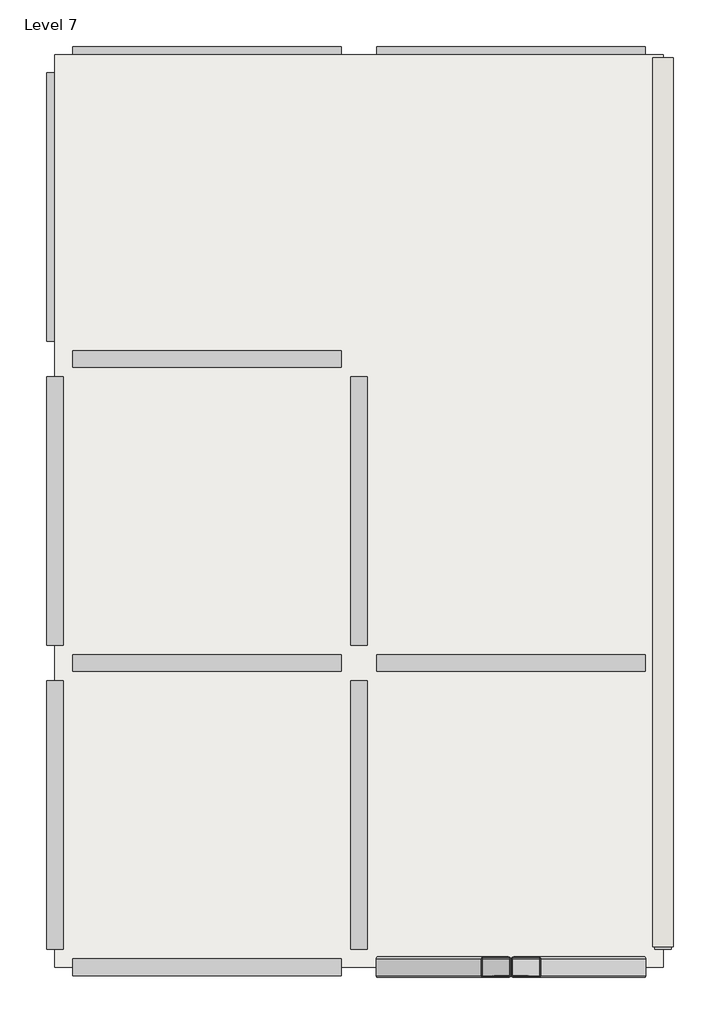
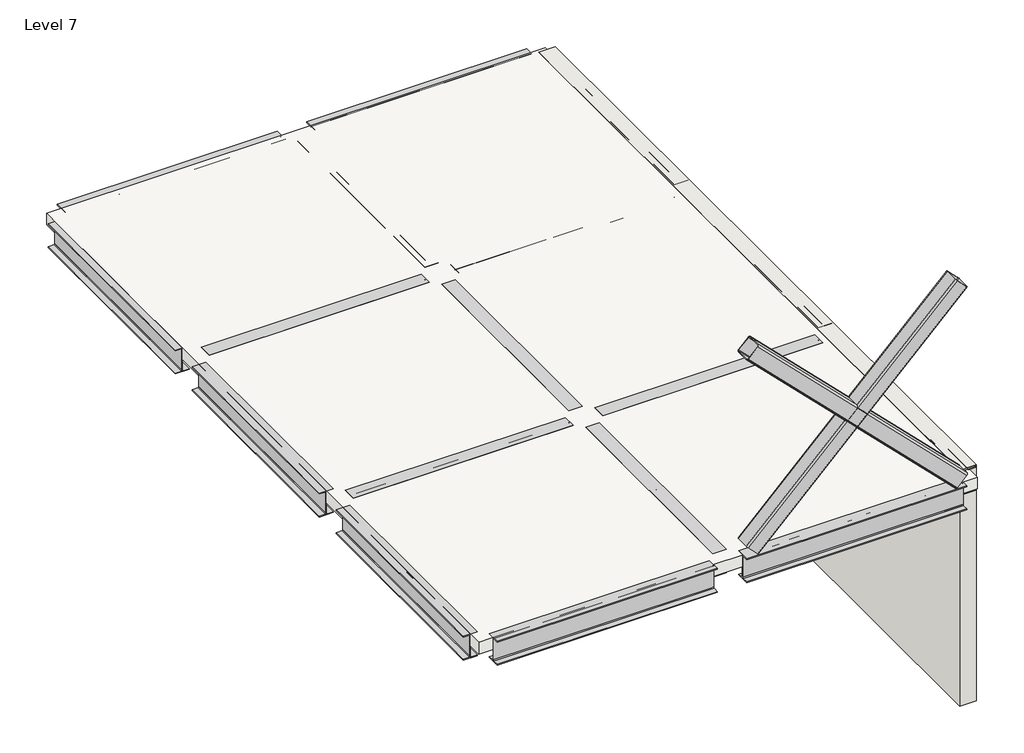
# One storey: 17 beams, 2 members, 1 slab, 1 wall.
"""IFC4 building model written with IfcOpenShell, lengths in millimetres."""

from ifc_helpers import new_model, si_unit, frame, origin, place, context, project, spatial, polyline, outline, extrude, transform, mapped, element, save
from components import ub_universal_beams_ub305x165x40_60ab2ee1, m_hss_square_hss203_2x203_2x9_5_07d005dd

model = new_model("IFC4")

# Units and contexts
model_context = context("Model", 3, world=origin())
ifc_project = project(units=[si_unit("LENGTHUNIT", "METRE", prefix="MILLI")], contexts=[model_context])

# Site, building, storey
site = spatial("IfcSite", under=ifc_project)
building = spatial("IfcBuilding", under=site)
storey = spatial("IfcBuildingStorey", under=building, Name="Level 7", Elevation=18000.0)

# Beams
placement = place(None, origin())
ub_universal_beams_ub305x165x40_shape = ub_universal_beams_ub305x165x40_60ab2ee1(model_context)
element("IfcBeam", 1, ObjectType="UB-Universal Beams : UB305x165x40", at=placement, inside=storey, context=model_context, shape_type="MappedRepresentation", body=[
    mapped(ub_universal_beams_ub305x165x40_shape, transform((18435.1404262, -6314.7314166, 17848.3), x_axis=(-1.0, 0.0, 0.0), y_axis=(0.0, -1.0, 0.0), z_axis=(0.0, 0.0, 1.0))),
])
element("IfcBeam", 2, ObjectType="UB-Universal Beams : UB305x165x40", at=placement, inside=storey, context=model_context, shape_type="MappedRepresentation", body=[
    mapped(ub_universal_beams_ub305x165x40_shape, transform((15435.1404262, -6314.7314166, 17848.3), x_axis=(-1.0, 0.0, 0.0), y_axis=(0.0, -1.0, 0.0), z_axis=(0.0, 0.0, 1.0))),
])
element("IfcBeam", 3, ObjectType="UB-Universal Beams : UB305x165x40", at=placement, inside=storey, context=model_context, shape_type="MappedRepresentation", body=[
    mapped(ub_universal_beams_ub305x165x40_shape, transform((13935.1404262, -4814.7314166, 17848.3), x_axis=(0.0, 1.0, 0.0), y_axis=(-1.0, 0.0, 0.0), z_axis=(0.0, 0.0, 1.0))),
])
element("IfcBeam", 4, ObjectType="UB-Universal Beams : UB305x165x40", at=placement, inside=storey, context=model_context, shape_type="MappedRepresentation", body=[
    mapped(ub_universal_beams_ub305x165x40_shape, transform((13935.1404262, -1814.7314166, 17848.3), x_axis=(0.0, 1.0, 0.0), y_axis=(-1.0, 0.0, 0.0), z_axis=(0.0, 0.0, 1.0))),
])
element("IfcBeam", 5, ObjectType="UB-Universal Beams : UB305x165x40", at=placement, inside=storey, context=model_context, shape_type="MappedRepresentation", body=[
    mapped(ub_universal_beams_ub305x165x40_shape, transform((13935.1404262, 1185.2685834, 17848.3), x_axis=(0.0, 1.0, 0.0), y_axis=(-1.0, 0.0, 0.0), z_axis=(0.0, 0.0, 1.0))),
])
element("IfcBeam", 6, ObjectType="UB-Universal Beams : UB305x165x40", at=placement, inside=storey, context=model_context, shape_type="MappedRepresentation", body=[
    mapped(ub_universal_beams_ub305x165x40_shape, transform((18435.1404262, -3314.7314166, 17848.3), x_axis=(-1.0, 0.0, 0.0), y_axis=(0.0, -1.0, 0.0), z_axis=(0.0, 0.0, 1.0))),
])
element("IfcBeam", 7, ObjectType="UB-Universal Beams : UB305x165x40", at=placement, inside=storey, context=model_context, shape_type="MappedRepresentation", body=[
    mapped(ub_universal_beams_ub305x165x40_shape, transform((15435.1404262, -3314.7314166, 17848.3), x_axis=(-1.0, 0.0, 0.0), y_axis=(0.0, -1.0, 0.0), z_axis=(0.0, 0.0, 1.0))),
])
element("IfcBeam", 8, ObjectType="UB-Universal Beams : UB305x165x40", at=placement, inside=storey, context=model_context, shape_type="MappedRepresentation", body=[
    mapped(ub_universal_beams_ub305x165x40_shape, transform((18435.1404262, -314.7314166, 17848.3), x_axis=(-1.0, 0.0, 0.0), y_axis=(0.0, -1.0, 0.0), z_axis=(0.0, 0.0, 1.0))),
])
element("IfcBeam", 9, ObjectType="UB-Universal Beams : UB305x165x40", at=placement, inside=storey, context=model_context, shape_type="MappedRepresentation", body=[
    mapped(ub_universal_beams_ub305x165x40_shape, transform((15435.1404262, -314.7314166, 17848.3), x_axis=(-1.0, 0.0, 0.0), y_axis=(0.0, -1.0, 0.0), z_axis=(0.0, 0.0, 1.0))),
])
element("IfcBeam", 10, ObjectType="UB-Universal Beams : UB305x165x40", at=placement, inside=storey, context=model_context, shape_type="MappedRepresentation", body=[
    mapped(ub_universal_beams_ub305x165x40_shape, transform((18435.1404262, 2685.2685834, 17848.3), x_axis=(-1.0, 0.0, 0.0), y_axis=(0.0, -1.0, 0.0), z_axis=(0.0, 0.0, 1.0))),
])
element("IfcBeam", 11, ObjectType="UB-Universal Beams : UB305x165x40", at=placement, inside=storey, context=model_context, shape_type="MappedRepresentation", body=[
    mapped(ub_universal_beams_ub305x165x40_shape, transform((15435.1404262, 2685.2685834, 17848.3), x_axis=(-1.0, 0.0, 0.0), y_axis=(0.0, -1.0, 0.0), z_axis=(0.0, 0.0, 1.0))),
])
element("IfcBeam", 12, ObjectType="UB-Universal Beams : UB305x165x40", at=placement, inside=storey, context=model_context, shape_type="MappedRepresentation", body=[
    mapped(ub_universal_beams_ub305x165x40_shape, transform((16935.1404262, -4814.7314166, 17848.3), x_axis=(0.0, 1.0, 0.0), y_axis=(-1.0, 0.0, 0.0), z_axis=(0.0, 0.0, 1.0))),
])
element("IfcBeam", 13, ObjectType="UB-Universal Beams : UB305x165x40", at=placement, inside=storey, context=model_context, shape_type="MappedRepresentation", body=[
    mapped(ub_universal_beams_ub305x165x40_shape, transform((16935.1404262, -1814.7314166, 17848.3), x_axis=(0.0, 1.0, 0.0), y_axis=(-1.0, 0.0, 0.0), z_axis=(0.0, 0.0, 1.0))),
])
element("IfcBeam", 14, ObjectType="UB-Universal Beams : UB305x165x40", at=placement, inside=storey, context=model_context, shape_type="MappedRepresentation", body=[
    mapped(ub_universal_beams_ub305x165x40_shape, transform((16935.1404262, 1185.2685834, 17848.3), x_axis=(0.0, 1.0, 0.0), y_axis=(-1.0, 0.0, 0.0), z_axis=(0.0, 0.0, 1.0))),
])
element("IfcBeam", 15, ObjectType="UB-Universal Beams : UB305x165x40", at=placement, inside=storey, context=model_context, shape_type="MappedRepresentation", body=[
    mapped(ub_universal_beams_ub305x165x40_shape, transform((19935.1404262, -1814.7314166, 17848.3), x_axis=(0.0, 1.0, 0.0), y_axis=(-1.0, 0.0, 0.0), z_axis=(0.0, 0.0, 1.0))),
])
element("IfcBeam", 16, ObjectType="UB-Universal Beams : UB305x165x40", at=placement, inside=storey, context=model_context, shape_type="MappedRepresentation", body=[
    mapped(ub_universal_beams_ub305x165x40_shape, transform((19935.1404262, 1185.2685834, 17848.3), x_axis=(0.0, 1.0, 0.0), y_axis=(-1.0, 0.0, 0.0), z_axis=(0.0, 0.0, 1.0))),
])
element("IfcBeam", 17, ObjectType="UB-Universal Beams : beam", at=placement, inside=storey, context=model_context, shape_type="MappedRepresentation", body=[
    mapped(ub_universal_beams_ub305x165x40_shape, transform((19935.1404262, -4814.7314166, 17848.3), x_axis=(0.0, 1.0, 0.0), y_axis=(-1.0, 0.0, 0.0), z_axis=(0.0, 0.0, 1.0))),
])

# Members
m_hss_square_hss203_2x203_2x9_5_shape = m_hss_square_hss203_2x203_2x9_5_07d005dd(model_context)
element("IfcMember", 18, ObjectType="M_HSS Square : HSS203.2X203.2X9.5", at=placement, inside=storey, context=model_context, shape_type="MappedRepresentation", body=[
    mapped(m_hss_square_hss203_2x203_2x9_5_shape, transform((18435.1404262, -6314.7314166, 19348.3), x_axis=(-0.7071067811865478, 0.0, 0.7071067811865476), y_axis=(0.0, -1.0000000000000002, 0.0), z_axis=(0.7071067811865476, 0.0, 0.7071067811865478))),
])
element("IfcMember", 19, ObjectType="M_HSS Square : HSS203.2X203.2X9.5", at=placement, inside=storey, context=model_context, shape_type="MappedRepresentation", body=[
    mapped(m_hss_square_hss203_2x203_2x9_5_shape, transform((18435.1404262, -6314.7314166, 19348.3), x_axis=(-0.7071067811865478, 0.0, -0.7071067811865475), y_axis=(0.0, -1.0000000000000002, 0.0), z_axis=(-0.7071067811865475, 0.0, 0.7071067811865478))),
])

# Slab
element("IfcSlab", 20, ObjectType="150mm Foundation Slab", at=placement, inside=storey, context=model_context, shape_type="SweptSolid", body=[
    extrude(outline(polyline([(13935.1404262, -6314.7314166), (13935.1404262, 2685.2685834), (19935.1404262, 2685.2685834), (19935.1404262, -6314.7314166), (13935.1404262, -6314.7314166)])), frame((0.0, 0.0, 17850.0), z_axis=(0.0, 0.0, 1.0), x_axis=(1.0, 0.0, 0.0)), (0.0, 0.0, 1.0), 150.0),
])

# Wall
element("IfcWall", 21, ObjectType="Generic - 200mm", at=placement, inside=storey, context=model_context, shape_type="SweptSolid", body=[
    extrude(outline(polyline([(19835.1404262, -6114.7314166), (19835.1404262, 2655.9792615), (20035.1404262, 2655.9792615), (20035.1404262, -6114.7314166), (19835.1404262, -6114.7314166)])), frame((0.0, 0.0, 15000.0), z_axis=(0.0, 0.0, 1.0), x_axis=(1.0, 0.0, 0.0)), (0.0, 0.0, 1.0), 3000.0),
])

save(model, "model.ifc")

# Revit data of these elements
# Type "UB-Universal Beams : UB305x165x40"
#   Section Name Key = "UB305X165X40"
#   Width = 16.5 cm
#   Web Thickness = 0.6 cm
#   Web Fillet = 0.89 cm
#   Warping Constant = 164000.0 cm⁶
#   Torsional Moment of Inertia = 14.70 cm⁴
#   Section Area = 51.3 cm²
#   Plastic Modulus weak axis = 142.0 cm³
#   Plastic Modulus strong axis = 623.0 cm³
#   Nominal Weight = 40.2999 kgf/m
#   Moment of Inertia weak axis = 764.00 cm⁴
#   Moment of Inertia strong axis = 8503.00 cm⁴
#   Height = 30.34 cm
#   Flange Thickness = 1.02 cm
#   Elastic Modulus weak axis = 92.6 cm³
#   Elastic Modulus strong axis = 560.0 cm³
#   Centroid Vertical = 15.17 cm
#   Centroid Horizontal = 8.25 cm
#   Bolt Spacing = 9.0 cm
#   Length [instance default] = 1.5 m
#   Structural Material [instance default] = Metal - Steel 43-275
#   Type Comments = ""
#   Assembly Code = ""
# Type "UB-Universal Beams : beam"
#   Section Name Key = "UB305X165X40"
#   Width = 16.5 cm
#   Web Thickness = 0.6 cm
#   Web Fillet = 0.89 cm
#   Warping Constant = 164000.0 cm⁶
#   Torsional Moment of Inertia = 14.70 cm⁴
#   Section Area = 51.3 cm²
#   Plastic Modulus weak axis = 142.0 cm³
#   Plastic Modulus strong axis = 623.0 cm³
#   Nominal Weight = 40.2999 kgf/m
#   Moment of Inertia weak axis = 764.00 cm⁴
#   Moment of Inertia strong axis = 8503.00 cm⁴
#   Height = 30.34 cm
#   Flange Thickness = 1.02 cm
#   Elastic Modulus weak axis = 92.6 cm³
#   Elastic Modulus strong axis = 560.0 cm³
#   Centroid Vertical = 15.17 cm
#   Centroid Horizontal = 8.25 cm
#   Bolt Spacing = 9.0 cm
#   Length [instance default] = 1.5 m
#   Structural Material [instance default] = Metal - Steel 43-275
#   Type Comments = ""
#   Assembly Code = ""
# Type "M_HSS Square : HSS203.2X203.2X9.5"
#   Section Name Key = "HSS 8X8X3/8"
#   Width = 20.3 cm
#   Wall Nominal Thickness = 0.953 cm
#   Wall Design Thickness = 0.886 cm
#   Torsional Moment of Inertia = 6660.00 cm⁴
#   Torsional Modulus = 10930171.7 cm³
#   Section Area = 67.1 cm²
#   Plastic Modulus weak axis = 482.0 cm³
#   Plastic Modulus strong axis = 482.0 cm³
#   Outer Fillet = 1.906 cm
#   Nominal Weight = 55.9998 kgf/m
#   Moment of Inertia weak axis = 4160.00 cm⁴
#   Moment of Inertia strong axis = 4160.00 cm⁴
#   Length [instance default] = 1.524 m
#   Inner Fillet = 0.953 cm
#   Height = 20.3 cm
#   Elastic Modulus weak axis = 408.0 cm³
#   Elastic Modulus strong axis = 408.0 cm³
#   Centroid Vertical = 10.15 cm
#   Centroid Horizontal = 10.15 cm
#   Structural Material [instance default] = Steel, 45-345
# Type "150mm Foundation Slab"
#   Layers, outside or top first: 0.15 m "Concrete, Cast-in-Place gray" (function 1)
# Type "Generic - 200mm"
#   Layers, outside or top first: 0.2 m no material (function 1)
# Elements 1, 2, 3, 4, 5, 6, 7, 8, 9, 10, 11, 12, 13, 14, 15, 16 (IfcBeam, "UB-Universal Beams : UB305x165x40")
#   Structural Material = Metal - Steel 43-275
#   Phase Created = New Construction
#   Materials on its faces: "Metal - Steel 43-275"
# Element 17 (IfcBeam, "UB-Universal Beams : beam")
#   Structural Material = Metal - Steel 43-275
#   Phase Created = New Construction
#   Materials on its faces: "Metal - Steel 43-275"
# Elements 18, 19 (IfcMember, "M_HSS Square : HSS203.2X203.2X9.5")
#   Comments = ""
#   Structural Material = Metal - Steel 43-275
#   Phase Created = New Construction
#   Materials on its faces: "Metal - Steel 43-275"
# Element 20 (IfcSlab, "150mm Foundation Slab")
#   built-in parameter 1001955 = 3.14159 (stored number, unit not read)
#   Height Offset From Level = 0 m
#   built-in parameter 1001954 = 1
#   Phase Created = New Construction
#   Materials on its faces: "Concrete, Cast-in-Place gray"
# Element 21 (IfcWall, "Generic - 200mm")
#   Comments = ""
#   built-in parameter 1001111 = -3 m
#   Top Offset = 0 m
#   Base Offset = -3 m
#   wall height = 3 m
#   Phase Created = New Construction
#   Base Constraint = Level 7
#   Top Constraint = Level 7
#   Materials on its faces: "Default Wall"
# Materials
#   "Metal - Steel 43-275": class "Metal", colour RGB 247 247 247, transparency 0, Cost = 0
#   "Steel, 45-345": class "Metal", colour RGB 247 247 247, transparency 0, Description = "Steel 345 MPa", Cost = 0
#   "Concrete, Cast-in-Place gray": class "Concrete", colour RGB 192 192 192, transparency 0, Description = "Cast-in-place concrete", Cost = 0
#   "Default Wall": colour RGB 128 128 128, transparency 0, Cost = 0
